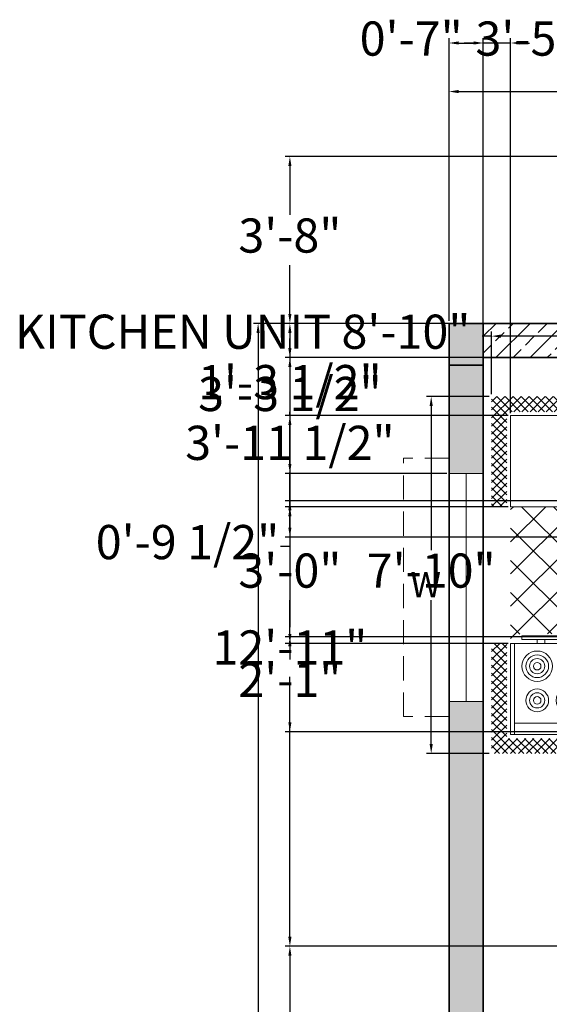
# Model space of a CAD drawing. Units: inches. Extents: x 9689 to 10369, y 10965 to 11626.
# Tile 5 of 11: x 9689 to 9828, y 11359 to 11619. Entities that reach past the tile are written whole.
import ezdxf

# ---------------------------------------------------------------- set-up
doc = ezdxf.new("R2010")
doc.units = ezdxf.units.IN
doc.linetypes.add('DASHED2', pattern=[9.525, 6.35, -3.175])
for name, color, linetype, lineweight in [('A-ANNO-DIMS', 2, 'Continuous', 18), ('A-ANNO-TEXT', 7, 'Continuous', 18), ('A-COLS', 7, 'Continuous', 35), ('A-FLOR-FIXT', 8, 'Continuous', 18), ('A-GLAZ', 4, 'Continuous', 18), ('A-GLAZ-OVHD', 4, 'DASHED2', 13), ('A-WALL', 7, 'Continuous', 35), ('A-WALL-PATT', 252, 'Continuous', 13)]:
    doc.layers.add(name, color=color, linetype=linetype, lineweight=lineweight)
doc.layers.add('A-COLS-PATT', color=18, linetype='Continuous', lineweight=13, true_color=0x000000)
doc.styles.get("Standard").update_dxf_attribs({"font": 'arial.ttf'})
doc.dimstyles.new('ISO-25', dxfattribs={"dimtxt": 9, "dimasz": 2.5, "dimexe": 1.25, "dimexo": 0.625, "dimgap": 2, "dimtad": 0, "dimtih": 1, "dimtoh": 1, "dimdec": 1, "dimlunit": 4, "dimtxsty": 'Standard', "dimcen": 2.5, "dimadec": 0, "dimazin": 0, "dimtfac": 0.5, "dimtdec": 1, "dimtmove": 0, "dimatfit": 3, "dimfxl": 1, "dimarcsym": 0})

# ---------------------------------------------------------------- blocks, each defined once
blk = doc.blocks.new('Kitchen Layout - 7 x 8 ft')
for p, q in [((-5, 81.32), (2.68, 89)), ((-5, 83.44), (0.56, 89)), ((-5, 85.56), (-1.56, 89)), ((-5, 87.68), (-3.68, 89)), ((-1, 84.97), (-5, 88.97)), ((1.09, 85), (-2.91, 89)), ((3.21, 85), (-0.79, 89)), ((0.81, 85), (4.81, 89)), ((5.34, 85), (1.34, 89)), ((2.93, 85), (6.93, 89)), ((7.46, 85), (3.46, 89)), ((5.05, 85), (9.05, 89)), ((9.58, 85), (5.58, 89)), ((7.17, 85), (11.17, 89)), ((11.7, 85), (7.7, 89)), ((9.29, 85), (13.29, 89)), ((13.82, 85), (9.82, 89)), ((11.41, 85), (15.41, 89)), ((15.94, 85), (11.94, 89)), ((13.53, 85), (17.53, 89)), ((18.06, 85), (14.06, 89)), ((15.65, 85), (19.65, 89)), ((20.18, 85), (16.18, 89)), ((17.78, 85), (21.78, 89)), ((22.31, 85), (18.31, 89)), ((19.9, 85), (23.9, 89)), ((24.43, 85), (20.43, 89)), ((22.02, 85), (26.02, 89)), ((26.55, 85), (22.55, 89)), ((24.14, 85), (28.14, 89)), ((28.67, 85), (24.67, 89)), ((26.26, 85), (30.26, 89)), ((30.79, 85), (26.79, 89)), ((28.38, 85), (32.38, 89)), ((32.91, 85), (28.91, 89)), ((30.5, 85), (34.5, 89)), ((35.03, 85), (31.03, 89)), ((32.63, 85), (36.63, 89)), ((37.16, 85), (33.16, 89)), ((34.75, 85), (38.75, 89)), ((39.28, 85), (35.28, 89)), ((36.87, 85), (40.87, 89)), ((41.4, 85), (37.4, 89)), ((38.99, 85), (42.99, 89)), ((43.52, 85), (39.52, 89)), ((41.11, 85), (45.11, 89)), ((45.64, 85), (41.64, 89)), ((43.23, 85), (47.23, 89)), ((47.76, 85), (43.76, 89)), ((45.35, 85), (49.35, 89)), ((49.88, 85), (45.88, 89)), ((47.47, 85), (51.47, 89)), ((52, 85), (48, 89)), ((49.6, 85), (53.6, 89)), ((54.13, 85), (50.13, 89)), ((51.72, 85), (55.72, 89)), ((56.25, 85), (52.25, 89)), ((53.84, 85), (57.84, 89)), ((58.37, 85), (54.37, 89)), ((55.96, 85), (59.96, 89)), ((60.49, 85), (56.49, 89)), ((58.08, 85), (62.08, 89)), ((62.61, 85), (58.61, 89)), ((60.2, 85), (64.2, 89)), ((64.73, 85), (60.73, 89)), ((62.32, 85), (66.32, 89)), ((66.85, 85), (62.85, 89)), ((64.45, 85), (68.45, 89)), ((68.97, 85), (64.97, 89)), ((66.57, 85), (70.57, 89)), ((71.1, 85), (67.1, 89)), ((68.69, 85), (72.69, 89)), ((73.22, 85), (69.22, 89)), ((70.81, 85), (74.81, 89)), ((75.34, 85), (71.34, 89)), ((72.93, 85), (76.93, 89)), ((77.46, 85), (73.46, 89)), ((75.05, 85), (79.05, 89)), ((79.58, 85), (75.58, 89)), ((77.17, 85), (81.17, 89)), ((81.7, 85), (77.7, 89)), ((79.29, 85), (83.29, 89)), ((83.82, 85), (79.82, 89)), ((81.42, 85), (85.42, 89)), ((85.95, 85), (81.95, 89)), ((83.54, 85), (87.54, 89)), ((88.07, 85), (84.07, 89)), ((85.66, 85), (89.66, 89)), ((90.19, 85), (86.19, 89)), ((87.78, 85), (91.78, 89)), ((92.31, 85), (88.31, 89)), ((89.9, 85), (93.9, 89)), ((94.43, 85), (90.43, 89)), ((92.02, 85), (96.02, 89)), ((96.55, 85), (92.55, 89)), ((94.14, 85), (98.14, 89)), ((101, 82.67), (94.67, 89)), ((96.27, 85), (100.27, 89)), ((101, 84.79), (96.79, 89)), ((101, 86.92), (98.92, 89)), ((-1, 82.85), (-5, 86.85)), ((97, 83.61), (101, 87.61)), ((-1, 80.73), (-5, 84.73)), ((-5, 79.19), (-1, 83.19)), ((34, 84), (96, 84)), ((34, 60), (34, 84)), ((96, 84), (96, 60)), ((97, 81.49), (101, 85.49)), ((101, 80.55), (97, 84.55)), ((97, 79.37), (101, 83.37)), ((-1, 78.61), (-5, 82.61)), ((-5, 77.07), (-1, 81.07)), ((-1, 76.49), (-5, 80.49)), ((74, 81), (95, 81)), ((101, 78.43), (97, 82.43)), ((97, 77.25), (101, 81.25)), ((-5, 74.95), (-1, 78.95)), ((-1, 74.36), (-5, 78.36)), ((101, 76.31), (97, 80.31)), ((97, 75.13), (101, 79.13)), ((101, 74.19), (97, 78.19)), ((-5, 72.83), (-1, 76.83)), ((-1, 72.24), (-5, 76.24)), ((97, 73.01), (101, 77.01)), ((101, 72.07), (97, 76.07)), ((-5, 70.71), (-1, 74.71)), ((-1, 70.12), (-5, 74.12)), ((-5, 68.59), (-1, 72.59)), ((97, 70.89), (101, 74.89)), ((101, 69.95), (97, 73.95)), ((97, 68.76), (101, 72.76)), ((-1, 68), (-5, 72)), ((-5, 66.47), (-1, 70.47)), ((101, 67.82), (97, 71.82)), ((97, 66.64), (101, 70.64)), ((-1, 65.88), (-5, 69.88)), ((-5, 64.35), (-1, 68.35)), ((-1, 63.76), (-5, 67.76)), ((101, 65.7), (97, 69.7)), ((97, 64.52), (101, 68.52)), ((101, 63.58), (97, 67.58)), ((-5, 62.22), (-1, 66.22)), ((-1, 61.64), (-5, 65.64)), ((97, 62.4), (101, 66.4)), ((101, 61.46), (97, 65.46)), ((-5, 60.1), (-1, 64.1)), ((-1, 59.52), (-5, 63.52)), ((97, 60.28), (101, 64.28)), ((100.34, 60), (97, 63.34)), ((-5, 57.98), (-1, 61.98)), ((-1, 57.39), (-5, 61.39)), ((-4.86, 56), (-1, 59.86)), ((96, 60), (34, 60)), ((80, 60), (80, 59)), ((82, 59), (82, 60)), ((87, 59), (87, 60)), ((89, 60), (89, 59)), ((98.22, 60), (97, 61.22)), ((98.84, 60), (101, 62.16)), ((100.96, 60), (101, 60.04)), ((-1.73, 56), (-5, 59.27)), ((-3.85, 56), (-5, 57.15)), ((-2.74, 56), (-1, 57.74)), ((10.4, 24), (45.9, 59.5)), ((18.88, 24), (54.38, 59.5)), ((27.37, 24), (62.87, 59.5)), ((33.03, 55.11), (37.41, 59.5)), ((67.71, 24), (33.68, 58.04)), ((35.85, 24), (71.35, 59.5)), ((76.2, 24), (40.7, 59.5)), ((44.34, 24), (77.84, 57.5)), ((84.68, 24), (49.18, 59.5)), ((52.82, 24), (86.32, 57.5)), ((93.17, 24), (57.67, 59.5)), ((61.31, 24), (96, 58.69)), ((96, 29.65), (66.15, 59.5)), ((96, 38.14), (76.64, 57.5)), ((96, 46.63), (85.13, 57.5)), ((96, 55.11), (93.57, 57.54)), ((0, 57), (33, 57)), ((0, 30.57), (24.43, 55)), ((0, 39.06), (15.94, 55)), ((0, 47.54), (7.46, 55)), ((1.91, 24), (32.91, 55)), ((33.77, 24), (2.77, 55)), ((42.26, 24), (11.26, 55)), ((50.74, 24), (19.74, 55)), ((59.23, 24), (28.23, 55)), ((31, 55), (31, 56)), ((32, 55), (31, 55)), ((32, 56), (32, 55)), ((25.29, 24), (0, 49.29)), ((69.79, 24), (96, 50.21)), ((78.28, 24), (96, 41.72)), ((16.8, 24), (0, 40.8)), ((8.32, 24), (0, 32.32)), ((86.76, 24), (96, 33.24)), ((-5, 21.92), (-2.92, 24)), ((-5, 19.8), (-1, 23.8)), ((-1, 21.33), (-3.67, 24)), ((-1, 23.45), (-1.55, 24)), ((0, 24), (96, 24)), ((0, 0), (0, 24)), ((95.25, 24), (96, 24.75)), ((96, 24), (96, 0)), ((97, 22.1), (98.9, 24)), ((97, 19.97), (101, 23.97)), ((101, 21.16), (98.16, 24)), ((101, 23.28), (100.28, 24)), ((-1, 19.21), (-5, 23.21)), ((-5, 17.68), (-1, 21.68)), ((-1, 17.09), (-5, 21.09)), ((101, 19.03), (97, 23.03)), ((97, 17.85), (101, 21.85)), ((101, 16.91), (97, 20.91)), ((-5, 15.55), (-1, 19.55)), ((-1, 14.97), (-5, 18.97)), ((47.25, 6.5), (47.25, 18.5)), ((48.75, 18.5), (48.75, 6.5)), ((97, 15.73), (101, 19.73)), ((101, 14.79), (97, 18.79)), ((-5, 13.43), (-1, 17.43)), ((-1, 12.85), (-5, 16.85)), ((97, 13.61), (101, 17.61)), ((101, 12.67), (97, 16.67)), ((-5, 11.31), (-1, 15.31)), ((-1, 10.73), (-5, 14.73)), ((-5, 9.19), (-1, 13.19)), ((97, 11.49), (101, 15.49)), ((101, 10.55), (97, 14.55)), ((97, 9.37), (101, 13.37)), ((-1, 8.6), (-5, 12.6)), ((-5, 7.07), (-1, 11.07)), ((-1, 6.48), (-5, 10.48)), ((101, 8.43), (97, 12.43)), ((97, 7.25), (101, 11.25)), ((-5, 4.95), (-1, 8.95)), ((-1, 4.36), (-5, 8.36)), ((101, 6.31), (97, 10.31)), ((97, 5.12), (101, 9.12)), ((101, 4.18), (97, 8.18)), ((-5, 2.83), (-1, 6.83)), ((-1, 2.24), (-5, 6.24)), ((97, 3), (101, 7)), ((101, 2.06), (97, 6.06)), ((-5, 0.71), (-1, 4.71)), ((-1, 0.12), (-5, 4.12)), ((64, 4), (32, 4)), ((93.24, -5), (101, 2.76)), ((97, 0.88), (101, 4.88)), ((101, -0.06), (97, 3.94)), ((-5, -1.42), (-1, 2.58)), ((2, -5), (-5, 2)), ((-5, -3.54), (-1, 0.46)), ((96, 0), (0, 0)), ((95.36, -5), (101, 0.64)), ((101, -2.18), (97, 1.82)), ((-0.12, -5), (-5, -0.12)), ((-2.25, -5), (-5, -2.25)), ((-4.34, -5), (-0.34, -1)), ((-2.22, -5), (1.78, -1)), ((-0.1, -5), (3.9, -1)), ((4.12, -5), (0.12, -1)), ((2.02, -5), (6.02, -1)), ((6.24, -5), (2.24, -1)), ((4.14, -5), (8.14, -1)), ((8.36, -5), (4.36, -1)), ((6.27, -5), (10.27, -1)), ((10.48, -5), (6.48, -1)), ((8.39, -5), (12.39, -1)), ((12.6, -5), (8.6, -1)), ((10.51, -5), (14.51, -1)), ((14.73, -5), (10.73, -1)), ((12.63, -5), (16.63, -1)), ((16.85, -5), (12.85, -1)), ((14.75, -5), (18.75, -1)), ((18.97, -5), (14.97, -1)), ((16.87, -5), (20.87, -1)), ((21.09, -5), (17.09, -1)), ((18.99, -5), (22.99, -1)), ((23.21, -5), (19.21, -1)), ((21.11, -5), (25.11, -1)), ((25.33, -5), (21.33, -1)), ((23.24, -5), (27.24, -1)), ((27.45, -5), (23.45, -1)), ((25.36, -5), (29.36, -1)), ((29.57, -5), (25.57, -1)), ((27.48, -5), (30, -2.48)), ((30, -3.3), (27.7, -1)), ((30, -1.18), (29.82, -1)), ((66, -2.54), (67.54, -1)), ((66, -4.66), (69.66, -1)), ((69.88, -5), (66, -1.12)), ((67.78, -5), (71.78, -1)), ((72, -5), (68, -1)), ((69.9, -5), (73.9, -1)), ((74.12, -5), (70.12, -1)), ((72.03, -5), (76.03, -1)), ((76.24, -5), (72.24, -1)), ((74.15, -5), (78.15, -1)), ((78.36, -5), (74.36, -1)), ((76.27, -5), (80.27, -1)), ((80.49, -5), (76.49, -1)), ((78.39, -5), (82.39, -1)), ((82.61, -5), (78.61, -1)), ((80.51, -5), (84.51, -1)), ((84.73, -5), (80.73, -1)), ((82.63, -5), (86.63, -1)), ((86.85, -5), (82.85, -1)), ((84.75, -5), (88.75, -1)), ((88.97, -5), (84.97, -1)), ((86.88, -5), (90.88, -1)), ((91.09, -5), (87.09, -1)), ((89, -5), (93, -1)), ((93.21, -5), (89.21, -1)), ((91.12, -5), (95.12, -1)), ((95.34, -5), (91.34, -1)), ((97.46, -5), (93.46, -1)), ((99.58, -5), (95.58, -1)), ((101, -4.3), (97, -0.3)), ((97.48, -5), (101, -1.48)), ((-4.37, -5), (-5, -4.37)), ((29.6, -5), (30, -4.6)), ((67.76, -5), (66, -3.24)), ((99.6, -5), (101, -3.6))]:
    blk.add_line(p, q)
for points in [[(0, 56), (0, 84), (33, 84), (33, 56)], [(74, 60), (74, 84), (95, 84), (95, 60)], [(76, 58), (76, 59), (93, 59), (93, 58)]]:
    blk.add_lwpolyline(points, close=True)
for points in [[(33.5, 21), (62.5, 21)], [(32, 1.5), (32, 19.5)], [(33.5, 6.5), (33.5, 18.5)], [(34.5, 19.5), (46.25, 19.5)], [(49.75, 19.5), (61.5, 19.5)], [(62.5, 18.5), (62.5, 6.5)], [(64, 19.5), (64, 1.5)], [(46.25, 5.5), (34.5, 5.5)], [(61.5, 5.5), (49.75, 5.5)], [(62.5, 0), (33.5, 0)]]:
    blk.add_lwpolyline(points)
for centre, radius in [((80, 75), 4), ((80, 75), 3), ((89, 75), 3), ((80, 75), 2), ((80, 75), 1), ((89, 75), 2), ((89, 75), 1), ((89, 66), 4), ((80, 66), 3), ((80, 66), 2), ((89, 66), 3), ((89, 66), 2), ((80, 66), 1), ((89, 66), 1), ((40.5, 12.5), 1), ((40.5, 12.5), 0.5), ((55.5, 12.5), 1), ((55.5, 12.5), 0.5)]:
    blk.add_circle(centre, radius)
for centre, radius, start, end in [((33.5, 19.5), 1.5, 90, 180), ((62.5, 19.5), 1.5, 0, 90), ((34.5, 18.5), 1, 90, 180), ((46.25, 18.5), 1, 0, 90), ((49.75, 18.5), 1, 90, 180), ((61.5, 18.5), 1, 0, 90), ((34.5, 6.5), 1, 180, 270), ((46.25, 6.5), 1, 270, 0), ((49.75, 6.5), 1, 180, 270), ((61.5, 6.5), 1, 270, 0), ((33.5, 1.5), 1.5, 180, 270), ((62.5, 1.5), 1.5, 270, 0)]:
    blk.add_arc(centre, radius, start, end)
blk = doc.blocks.new('*D20')
at = {"layer": 'A-ANNO-DIMS', "color": 0, "lineweight": -2, "transparency": 16777216}
for p, q in [((9801.43, 11538.63), (9750.54, 11538.63)), ((9751.79, 11536.13), (9751.79, 11280.15)), ((9751.79, 11011.13), (9751.79, 11267.11)), ((9801.43, 11008.63), (9750.54, 11008.63))]:
    blk.add_line(p, q, dxfattribs=at)
at = {"layer": 'A-ANNO-DIMS', "color": 0, "transparency": 16777216}
for points in [[(9751.38, 11536.13), (9752.21, 11536.13), (9751.79, 11538.63)], [(9751.38, 11011.13), (9752.21, 11011.13), (9751.79, 11008.63)]]:
    blk.add_solid(points, dxfattribs=at)
at = {"layer": 'Defpoints', "color": 0, "transparency": 16777216}
for p in [(9802.06, 11538.63), (9751.79, 11008.63), (9802.06, 11008.63)]:
    blk.add_point(p, dxfattribs=at)
at = {"layer": 'A-ANNO-DIMS', "color": 0, "transparency": 16777216, "insert": (9751.79, 11273.63), "char_height": 9, "attachment_point": 5}
blk.add_mtext('44\'-2"', dxfattribs=at)
blk = doc.blocks.new('*D21')
at = {"layer": 'A-ANNO-DIMS', "color": 0, "lineweight": -2, "transparency": 16777216}
for p, q in [((9802.06, 11539.26), (9802.06, 11600.92)), ((10244.06, 11539.26), (10244.06, 11600.92)), ((9804.56, 11599.67), (10002.11, 11599.67)), ((10241.56, 11599.67), (10044.01, 11599.67))]:
    blk.add_line(p, q, dxfattribs=at)
at = {"layer": 'A-ANNO-DIMS', "color": 0, "transparency": 16777216}
for points in [[(9804.56, 11600.08), (9804.56, 11599.25), (9802.06, 11599.67)], [(10241.56, 11600.08), (10241.56, 11599.25), (10244.06, 11599.67)]]:
    blk.add_solid(points, dxfattribs=at)
at = {"layer": 'Defpoints', "color": 0, "transparency": 16777216}
for p in [(10244.06, 11599.67), (9802.06, 11538.63), (10244.06, 11538.63)]:
    blk.add_point(p, dxfattribs=at)
at = {"layer": 'A-ANNO-DIMS', "color": 0, "transparency": 16777216, "insert": (10023.06, 11599.67), "char_height": 9, "attachment_point": 5}
blk.add_mtext('36\'-10"', dxfattribs=at)
blk = doc.blocks.new('WINDOW-HOOD-68')
for p, q in [((12, 68), (0, 68)), ((0, 0), (0, 68)), ((12, 0), (0, 0))]:
    blk.add_line(p, q)
blk = doc.blocks.new('WINDOW-60')
for p, q in [((0, 60), (9, 60)), ((4.5, 60), (4.5, 0)), ((0, 0), (9, 0))]:
    blk.add_line(p, q)
blk = doc.blocks.new('*D50')
at = {"layer": 'A-ANNO-DIMS', "color": 0, "lineweight": -2, "transparency": 16777216}
for p, q in [((9813.25, 11519.99), (9813.25, 11536.52)), ((9919.25, 11519.99), (9919.25, 11536.52)), ((9813.25, 11535.27), (9810.75, 11535.27)), ((9916.75, 11535.27), (9815.75, 11535.27))]:
    blk.add_line(p, q, dxfattribs=at)
at = {"layer": 'A-ANNO-DIMS', "color": 0, "transparency": 16777216}
for points in [[(9815.75, 11535.69), (9815.75, 11534.85), (9813.25, 11535.27)], [(9916.75, 11535.69), (9916.75, 11534.85), (9919.25, 11535.27)]]:
    blk.add_solid(points, dxfattribs=at)
at = {"layer": 'Defpoints', "color": 0, "transparency": 16777216}
for p in [(9813.25, 11535.27), (9813.25, 11519.37), (9919.25, 11519.37)]:
    blk.add_point(p, dxfattribs=at)
at = {"layer": 'A-ANNO-DIMS', "color": 0, "transparency": 16777216, "insert": (9747.74, 11535.27), "char_height": 9, "attachment_point": 5}
blk.add_mtext('KITCHEN UNIT 8\'-10"', dxfattribs=at)
blk = doc.blocks.new('*D51')
at = {"layer": 'A-ANNO-DIMS', "color": 0, "lineweight": -2, "transparency": 16777216}
for p, q in [((9812.62, 11519.37), (9796.1, 11519.37)), ((9797.35, 11516.87), (9797.35, 11478.96)), ((9797.35, 11427.87), (9797.35, 11465.77)), ((9812.62, 11425.37), (9796.1, 11425.37))]:
    blk.add_line(p, q, dxfattribs=at)
at = {"layer": 'A-ANNO-DIMS', "color": 0, "transparency": 16777216}
for points in [[(9796.93, 11516.87), (9797.77, 11516.87), (9797.35, 11519.37)], [(9796.93, 11427.87), (9797.77, 11427.87), (9797.35, 11425.37)]]:
    blk.add_solid(points, dxfattribs=at)
at = {"layer": 'Defpoints', "color": 0, "transparency": 16777216}
for p in [(9813.25, 11519.37), (9797.35, 11425.37), (9813.25, 11425.37)]:
    blk.add_point(p, dxfattribs=at)
at = {"layer": 'A-ANNO-DIMS', "color": 0, "transparency": 16777216, "insert": (9797.35, 11472.37), "char_height": 9, "attachment_point": 5}
blk.add_mtext('7\'-10"', dxfattribs=at)
blk = doc.blocks.new('*D80')
at = {"layer": 'A-ANNO-DIMS', "color": 0, "lineweight": -2, "transparency": 16777216}
for p, q in [((9979.43, 11529.63), (9758.91, 11529.63)), ((9760.16, 11527.13), (9760.16, 11512.66)), ((9760.16, 11484.88), (9760.16, 11499.35)), ((9979.43, 11482.38), (9758.91, 11482.38))]:
    blk.add_line(p, q, dxfattribs=at)
at = {"layer": 'A-ANNO-DIMS', "color": 0, "transparency": 16777216}
for points in [[(9759.74, 11527.13), (9760.57, 11527.13), (9760.16, 11529.63)], [(9759.74, 11484.88), (9760.57, 11484.88), (9760.16, 11482.38)]]:
    blk.add_solid(points, dxfattribs=at)
at = {"layer": 'Defpoints', "color": 0, "transparency": 16777216}
for p in [(9760.16, 11529.63), (9980.06, 11529.63), (9980.06, 11482.38)]:
    blk.add_point(p, dxfattribs=at)
at = {"layer": 'A-ANNO-DIMS', "color": 0, "transparency": 16777216, "insert": (9760.16, 11506.01), "char_height": 9, "attachment_point": 5}
blk.add_mtext('3\'-11 1/2"', dxfattribs=at)
blk = doc.blocks.new('*D82')
at = {"layer": 'A-ANNO-DIMS', "color": 0, "lineweight": -2, "transparency": 16777216}
for p, q in [((9898.43, 11582.55), (9758.91, 11582.55)), ((9760.16, 11580.05), (9760.16, 11567.19)), ((9760.16, 11541.13), (9760.16, 11553.99)), ((9898.43, 11538.63), (9758.91, 11538.63))]:
    blk.add_line(p, q, dxfattribs=at)
at = {"layer": 'A-ANNO-DIMS', "color": 0, "transparency": 16777216}
for points in [[(9759.74, 11580.05), (9760.57, 11580.05), (9760.16, 11582.55)], [(9759.74, 11541.13), (9760.57, 11541.13), (9760.16, 11538.63)]]:
    blk.add_solid(points, dxfattribs=at)
at = {"layer": 'Defpoints', "color": 0, "transparency": 16777216}
for p in [(9760.16, 11582.55), (9899.06, 11582.55), (9899.06, 11538.63)]:
    blk.add_point(p, dxfattribs=at)
at = {"layer": 'A-ANNO-DIMS', "color": 0, "transparency": 16777216, "insert": (9760.16, 11560.59), "char_height": 9, "attachment_point": 5}
blk.add_mtext('3\'-8"', dxfattribs=at)
blk = doc.blocks.new('*D86')
at = {"layer": 'A-ANNO-DIMS', "color": 0, "lineweight": -2, "transparency": 16777216}
for p, q in [((9802.06, 11539.26), (9802.06, 11613.7)), ((9804.56, 11612.45), (9808.6, 11612.45)), ((9840.56, 11612.45), (9836.52, 11612.45)), ((9843.06, 11539.26), (9843.06, 11613.7))]:
    blk.add_line(p, q, dxfattribs=at)
at = {"layer": 'A-ANNO-DIMS', "color": 0, "transparency": 16777216}
for points in [[(9804.56, 11612.87), (9804.56, 11612.04), (9802.06, 11612.45)], [(9840.56, 11612.87), (9840.56, 11612.04), (9843.06, 11612.45)]]:
    blk.add_solid(points, dxfattribs=at)
at = {"layer": 'Defpoints', "color": 0, "transparency": 16777216}
for p in [(9843.06, 11612.45), (9802.06, 11538.63), (9843.06, 11538.63)]:
    blk.add_point(p, dxfattribs=at)
at = {"layer": 'A-ANNO-DIMS', "color": 0, "transparency": 16777216, "insert": (9822.56, 11612.45), "char_height": 9, "attachment_point": 5}
blk.add_mtext('3\'-5"', dxfattribs=at)
blk = doc.blocks.new('*D91')
at = {"layer": 'A-ANNO-DIMS', "color": 0, "lineweight": -2, "transparency": 16777216}
for p, q in [((9801.43, 11538.63), (9758.91, 11538.63)), ((9760.16, 11536.13), (9760.16, 11525.53)), ((9760.16, 11501.61), (9760.16, 11512.22)), ((9801.43, 11499.11), (9758.91, 11499.11))]:
    blk.add_line(p, q, dxfattribs=at)
at = {"layer": 'A-ANNO-DIMS', "color": 0, "transparency": 16777216}
for points in [[(9759.74, 11536.13), (9760.57, 11536.13), (9760.16, 11538.63)], [(9759.74, 11501.61), (9760.57, 11501.61), (9760.16, 11499.11)]]:
    blk.add_solid(points, dxfattribs=at)
at = {"layer": 'Defpoints', "color": 0, "transparency": 16777216}
for p in [(9760.16, 11538.63), (9802.06, 11538.63), (9802.06, 11499.11)]:
    blk.add_point(p, dxfattribs=at)
at = {"layer": 'A-ANNO-DIMS', "color": 0, "transparency": 16777216, "insert": (9760.16, 11518.87), "char_height": 9, "attachment_point": 5}
blk.add_mtext('3\'-3 1/2"', dxfattribs=at)
blk = doc.blocks.new('*D99')
at = {"layer": 'A-ANNO-DIMS', "color": 0, "lineweight": -2, "transparency": 16777216}
for p, q in [((9922.43, 11374.63), (9758.91, 11374.63)), ((9760.16, 11372.13), (9760.16, 11357.23)), ((9760.16, 11329.13), (9760.16, 11344.03)), ((9801.43, 11326.63), (9758.91, 11326.63))]:
    blk.add_line(p, q, dxfattribs=at)
at = {"layer": 'A-ANNO-DIMS', "color": 0, "transparency": 16777216}
for points in [[(9759.74, 11372.13), (9760.57, 11372.13), (9760.16, 11374.63)], [(9759.74, 11329.13), (9760.57, 11329.13), (9760.16, 11326.63)]]:
    blk.add_solid(points, dxfattribs=at)
at = {"layer": 'Defpoints', "color": 0, "transparency": 16777216}
for p in [(9923.06, 11374.63), (9760.16, 11326.63), (9802.06, 11326.63)]:
    blk.add_point(p, dxfattribs=at)
at = {"layer": 'A-ANNO-DIMS', "color": 0, "transparency": 16777216, "insert": (9760.16, 11350.63), "char_height": 9, "attachment_point": 5}
blk.add_mtext('4\'-0"', dxfattribs=at)
blk = doc.blocks.new('*D108')
at = {"layer": 'A-ANNO-DIMS', "color": 0, "lineweight": -2, "transparency": 16777216}
for p, q in [((9922.43, 11529.63), (9758.91, 11529.63)), ((9760.16, 11527.13), (9760.16, 11458.65)), ((9760.16, 11377.13), (9760.16, 11445.61)), ((9922.43, 11374.63), (9758.91, 11374.63))]:
    blk.add_line(p, q, dxfattribs=at)
at = {"layer": 'A-ANNO-DIMS', "color": 0, "transparency": 16777216}
for points in [[(9759.74, 11527.13), (9760.57, 11527.13), (9760.16, 11529.63)], [(9759.74, 11377.13), (9760.57, 11377.13), (9760.16, 11374.63)]]:
    blk.add_solid(points, dxfattribs=at)
at = {"layer": 'Defpoints', "color": 0, "transparency": 16777216}
for p in [(9760.16, 11529.63), (9923.06, 11529.63), (9923.06, 11374.63)]:
    blk.add_point(p, dxfattribs=at)
at = {"layer": 'A-ANNO-DIMS', "color": 0, "transparency": 16777216, "insert": (9760.16, 11452.13), "char_height": 9, "attachment_point": 5}
blk.add_mtext('12\'-11"', dxfattribs=at)
blk = doc.blocks.new('*D110')
at = {"layer": 'A-ANNO-DIMS', "color": 0, "lineweight": -2, "transparency": 16777216}
for p, q in [((10021.43, 11456.13), (9758.91, 11456.13)), ((9760.16, 11453.63), (9760.16, 11450.15)), ((9760.16, 11433.63), (9760.16, 11437.11)), ((10021.43, 11431.13), (9758.91, 11431.13))]:
    blk.add_line(p, q, dxfattribs=at)
at = {"layer": 'A-ANNO-DIMS', "color": 0, "transparency": 16777216}
for points in [[(9759.74, 11453.63), (9760.57, 11453.63), (9760.16, 11456.13)], [(9759.74, 11433.63), (9760.57, 11433.63), (9760.16, 11431.13)]]:
    blk.add_solid(points, dxfattribs=at)
at = {"layer": 'Defpoints', "color": 0, "transparency": 16777216}
for p in [(9760.16, 11456.13), (10022.06, 11456.13), (10022.06, 11431.13)]:
    blk.add_point(p, dxfattribs=at)
at = {"layer": 'A-ANNO-DIMS', "color": 0, "transparency": 16777216, "insert": (9760.16, 11443.63), "char_height": 9, "attachment_point": 5}
blk.add_mtext('2\'-1"', dxfattribs=at)
blk = doc.blocks.new('*D114')
at = {"layer": 'A-ANNO-DIMS', "color": 0, "lineweight": -2, "transparency": 16777216}
for p, q in [((9817.62, 11490.37), (9758.91, 11490.37)), ((9760.16, 11487.87), (9760.16, 11478.97)), ((9760.16, 11456.87), (9760.16, 11465.77)), ((9817.62, 11454.37), (9758.91, 11454.37))]:
    blk.add_line(p, q, dxfattribs=at)
at = {"layer": 'A-ANNO-DIMS', "color": 0, "transparency": 16777216}
for points in [[(9759.74, 11487.87), (9760.57, 11487.87), (9760.16, 11490.37)], [(9759.74, 11456.87), (9760.57, 11456.87), (9760.16, 11454.37)]]:
    blk.add_solid(points, dxfattribs=at)
at = {"layer": 'Defpoints', "color": 0, "transparency": 16777216}
for p in [(9760.16, 11490.37), (9818.25, 11490.37), (9818.25, 11454.37)]:
    blk.add_point(p, dxfattribs=at)
at = {"layer": 'A-ANNO-DIMS', "color": 0, "transparency": 16777216, "insert": (9760.16, 11472.37), "char_height": 9, "attachment_point": 5}
blk.add_mtext('3\'-0"', dxfattribs=at)
blk = doc.blocks.new('*D115')
at = {"layer": 'A-ANNO-DIMS', "color": 0, "lineweight": -2, "transparency": 16777216}
for p, q in [((9760.16, 11532.13), (9760.16, 11534.63)), ((9810.43, 11529.63), (9758.91, 11529.63)), ((9760.16, 11529.63), (9760.16, 11528.66)), ((9817.62, 11514.37), (9758.91, 11514.37)), ((9760.16, 11514.37), (9760.16, 11515.34)), ((9760.16, 11511.87), (9760.16, 11509.37))]:
    blk.add_line(p, q, dxfattribs=at)
at = {"layer": 'A-ANNO-DIMS', "color": 0, "transparency": 16777216}
for points in [[(9759.74, 11532.13), (9760.57, 11532.13), (9760.16, 11529.63)], [(9759.74, 11511.87), (9760.57, 11511.87), (9760.16, 11514.37)]]:
    blk.add_solid(points, dxfattribs=at)
at = {"layer": 'Defpoints', "color": 0, "transparency": 16777216}
for p in [(9760.16, 11529.63), (9811.06, 11529.63), (9818.25, 11514.37)]:
    blk.add_point(p, dxfattribs=at)
at = {"layer": 'A-ANNO-DIMS', "color": 0, "transparency": 16777216, "insert": (9760.16, 11522), "char_height": 9, "attachment_point": 5}
blk.add_mtext('1\'-3 1/2"', dxfattribs=at)
blk = doc.blocks.new('*D116')
at = {"layer": 'A-ANNO-DIMS', "color": 0, "lineweight": -2, "transparency": 16777216}
for p, q in [((9808.56, 11612.45), (9806.06, 11612.45)), ((9811.06, 11530.26), (9811.06, 11613.7)), ((9818.25, 11612.45), (9811.06, 11612.45)), ((9818.25, 11514.99), (9818.25, 11613.7)), ((9820.75, 11612.45), (9823.25, 11612.45))]:
    blk.add_line(p, q, dxfattribs=at)
at = {"layer": 'A-ANNO-DIMS', "color": 0, "transparency": 16777216}
for points in [[(9808.56, 11612.87), (9808.56, 11612.04), (9811.06, 11612.45)], [(9820.75, 11612.87), (9820.75, 11612.04), (9818.25, 11612.45)]]:
    blk.add_solid(points, dxfattribs=at)
at = {"layer": 'Defpoints', "color": 0, "transparency": 16777216}
for p in [(9811.06, 11612.45), (9811.06, 11529.63), (9818.25, 11514.37)]:
    blk.add_point(p, dxfattribs=at)
at = {"layer": 'A-ANNO-DIMS', "color": 0, "transparency": 16777216, "insert": (9792.09, 11612.45), "char_height": 9, "attachment_point": 5}
blk.add_mtext('0\'-7"', dxfattribs=at)
blk = doc.blocks.new('*D118')
at = {"layer": 'A-ANNO-DIMS', "color": 0, "lineweight": -2, "transparency": 16777216}
for p, q in [((9980.91, 11491.91), (9758.91, 11491.91)), ((9760.16, 11489.41), (9760.16, 11484.88)), ((9979.43, 11482.38), (9758.91, 11482.38)), ((9760.16, 11482.38), (9760.16, 11479.88)), ((9760.16, 11479.88), (9757.66, 11479.88))]:
    blk.add_line(p, q, dxfattribs=at)
at = {"layer": 'A-ANNO-DIMS', "color": 0, "transparency": 16777216}
for points in [[(9759.74, 11489.41), (9760.57, 11489.41), (9760.16, 11491.91)], [(9759.74, 11484.88), (9760.57, 11484.88), (9760.16, 11482.38)]]:
    blk.add_solid(points, dxfattribs=at)
at = {"layer": 'Defpoints', "color": 0, "transparency": 16777216}
for p in [(9981.53, 11491.91), (9760.16, 11482.38), (9980.06, 11482.38)]:
    blk.add_point(p, dxfattribs=at)
at = {"layer": 'A-ANNO-DIMS', "color": 0, "transparency": 16777216, "insert": (9733.21, 11479.88), "char_height": 9, "attachment_point": 5}
blk.add_mtext('0\'-9 1/2"', dxfattribs=at)

msp = doc.modelspace()

# ---------------------------------------------------------------- hatches: boundary and pattern name
at = {"layer": 'A-COLS-PATT'}
h = msp.add_hatch(color=256, dxfattribs=at)
h.dxf.hatch_style = 1
h.paths.add_polyline_path([(9811.06, 11538.63), (9802.06, 11538.63), (9802.06, 11527.63), (9811.06, 11527.63), (9811.06, 11529.63)])
at = {"layer": 'A-WALL-PATT'}
h = msp.add_hatch(dxfattribs=at)
h.set_pattern_fill('ANSI33', color=256)
h.paths.add_polyline_path([(9843.06, 11538.63), (9811.06, 11538.63), (9811.06, 11529.63), (9843.06, 11529.63)])
h.paths.add_polyline_path([(9923.06, 11538.63), (9891.06, 11538.63), (9891.06, 11529.63), (9923.06, 11529.63)])
h.paths.add_polyline_path([(9929.06, 11527.63), (9923.06, 11527.63), (9923.06, 11380.63), (9929.06, 11380.63)])
h.paths.add_polyline_path([(9939.06, 11538.63), (9929.06, 11538.63), (9929.06, 11529.63), (9939.06, 11529.63, -0.071068)])
h.paths.add_polyline_path([(10035.06, 11538.63), (10013.06, 11538.63), (10013.06, 11529.63), (10022.06, 11529.63), (10022.06, 11507.38), (10022.06, 11502.38), (10022.06, 11482.38), (10022.06, 11478.38), (10022.06, 11456.13, -0.038405), (10026.06, 11456.13), (10026.06, 11502.38), (10026.06, 11529.63), (10035.06, 11529.63)])
h.paths.add_polyline_path([(10068.06, 11538.63), (10059.06, 11538.63), (10059.06, 11529.63), (10068.06, 11529.63)])
h.paths.add_polyline_path([(10074.06, 11527.63), (10068.06, 11527.63), (10068.06, 11431.13), (10026.06, 11431.13), (10022.06, 11431.13), (9980.06, 11431.13), (9976.06, 11431.13), (9976.06, 11425.13), (10068.06, 11425.13), (10068.06, 11380.63), (10074.06, 11380.63)])
h.paths.add_polyline_path([(10124.56, 11538.63), (10074.06, 11538.63), (10074.06, 11529.63), (10124.56, 11529.63)])
h.paths.add_polyline_path([(9980.06, 11507.38), (9980.06, 11529.63), (9989.06, 11529.63), (9989.06, 11538.63), (9976.06, 11538.63), (9976.06, 11529.63), (9976.06, 11503.38), (9976.06, 11483.38), (9976.06, 11478.38), (9980.06, 11478.38), (9997.06, 11478.38, -0.038405), (9997.06, 11482.38), (9980.06, 11482.38)])
h.paths.add_polyline_path([(10235.06, 11538.63), (10184.56, 11538.63), (10184.56, 11529.63), (10235.06, 11529.63)])
h.paths.add_polyline_path([(10244.06, 11527.63), (10235.06, 11527.63), (10235.06, 11485.13), (10244.06, 11485.13)])
h.paths.add_polyline_path([(10244.06, 11425.13), (10235.06, 11425.13), (10235.06, 11380.63), (10244.06, 11380.63)])
h.paths.add_polyline_path([(10233.06, 11380.63), (10120.06, 11380.63, -0.038405), (10120.06, 11374.63), (10133.04, 11374.63), (10133.04, 11326.63), (10120.06, 11326.63, -0.038405), (10120.06, 11320.63), (10149.19, 11320.63), (10149.19, 11326.63), (10136.04, 11326.63), (10136.04, 11374.63), (10233.06, 11374.63)])
h.paths.add_polyline_path([(10084.06, 11380.63), (10076.06, 11380.63), (10076.06, 11374.63), (10084.06, 11374.63)])
h.paths.add_polyline_path([(10244.06, 11374.63), (10235.06, 11374.63), (10235.06, 11362.63), (10244.06, 11362.63)])
h.paths.add_polyline_path([(10244.06, 11338.63), (10235.06, 11338.63), (10235.06, 11326.63), (10244.06, 11326.63)])
h.paths.add_polyline_path([(10233.06, 11326.63), (10173.19, 11326.63, -0.055385), (10173.19, 11320.63), (10233.06, 11320.63)], flags=0)
h.paths.add_polyline_path([(10244.06, 11320.63), (10235.06, 11320.63), (10235.06, 11273.63), (10244.06, 11273.63)])
h = msp.add_hatch(dxfattribs=at)
h.set_pattern_fill('ANSI36', color=256)
h.paths.add_polyline_path([(10233.06, 11326.63), (10173.19, 11326.63, -0.055385), (10173.19, 11320.63), (10233.06, 11320.63)])
h.paths.add_polyline_path([(10244.06, 11213.63), (10235.06, 11213.63), (10235.06, 11166.63), (10244.06, 11166.63)])
h.paths.add_polyline_path([(10233.06, 11166.63), (10184.56, 11166.63), (10184.56, 11157.63), (10233.06, 11157.63)])
h.paths.add_polyline_path([(10124.56, 11166.63), (10074.06, 11166.63), (10074.06, 11157.63), (10124.56, 11157.63)])
h.paths.add_polyline_path([(10074.06, 11318.63), (10068.06, 11318.63), (10068.06, 11168.63), (10074.06, 11168.63)])
h.paths.add_polyline_path([(10068.06, 11166.63), (10011.06, 11166.63), (10011.06, 11157.63), (10068.06, 11157.63)])
h.paths.add_polyline_path([(10011.06, 11318.63), (10005.06, 11318.63), (10005.06, 11168.63), (10011.06, 11168.63)])
h.paths.add_polyline_path([(10005.06, 11166.63), (9985.06, 11166.63), (9985.06, 11157.63), (10005.06, 11157.63)])
h.paths.add_polyline_path([(9937.06, 11166.63), (9898.06, 11166.63), (9898.06, 11157.63), (9937.06, 11157.63, -0.042779)])
h.paths.add_polyline_path([(9850.06, 11166.63), (9813.06, 11166.63), (9813.06, 11157.63), (9850.06, 11157.63)])
h.paths.add_polyline_path([(9811.06, 11213.63), (9802.06, 11213.63), (9802.06, 11166.63), (9811.06, 11166.63)])
h.paths.add_polyline_path([(9811.06, 11320.63), (9802.06, 11320.63), (9802.06, 11273.63), (9811.06, 11273.63)])
h.paths.add_polyline_path([(9811.06, 11439.11), (9802.06, 11439.11), (9802.06, 11326.63), (9811.06, 11326.63)])
h.paths.add_polyline_path([(9957.06, 11326.63), (9813.06, 11326.63), (9813.06, 11320.63), (9957.06, 11320.63)])
h.paths.add_polyline_path([(9811.06, 11527.63), (9802.06, 11527.63), (9802.06, 11499.11), (9811.06, 11499.11)])

# ---------------------------------------------------------------- linework, layer by layer
at = {"layer": 'A-COLS'}
for p, q in [((9811.06, 11529.63), (9811.06, 11538.63)), ((9811.06, 11527.63), (9802.06, 11527.63))]:
    msp.add_line(p, q, dxfattribs=at)
at = {"layer": 'A-GLAZ'}
msp.add_line((9811.06, 11499.11), (9811.06, 11439.11), dxfattribs=at)
at = {"layer": 'A-WALL'}
for p, q in [((9802.06, 11538.63), (9939.06, 11538.63)), ((9802.06, 11157.63), (9802.06, 11538.63)), ((9811.06, 11529.63), (9923.06, 11529.63)), ((9811.06, 11326.63), (9811.06, 11529.63))]:
    msp.add_line(p, q, dxfattribs=at)

# ---------------------------------------------------------------- block references
at = {"layer": 'A-FLOR-FIXT', "rotation": 180}
msp.add_blockref('Kitchen Layout - 7 x 8 ft', (9914.25, 11514.37), dxfattribs=at)
at = {"layer": 'A-GLAZ'}
msp.add_blockref('WINDOW-60', (9802.06, 11439.11), dxfattribs=at)
at = {"layer": 'A-GLAZ-OVHD'}
msp.add_blockref('WINDOW-HOOD-68', (9790.06, 11435.11), dxfattribs=at)

# ---------------------------------------------------------------- texts
at = {"layer": 'A-ANNO-TEXT', "insert": (9791.89, 11473.21), "char_height": 6.729, "attachment_point": 1}
msp.add_mtext_dynamic_manual_height_columns('{\\fArial|b1|i0|c0|p34;W}', width=31.3623, gutter_width=33.65, heights=[0], dxfattribs=at)

# ---------------------------------------------------------------- dimensions: what is measured, and where the dimension line sits
at = {"layer": 'A-ANNO-DIMS'}
for base, p1, p2, override, picture, middle in [((9811.06, 11612.45), (9818.25, 11514.37), (9811.06, 11529.63), {"dimdec": 1, "dimlfac": 1, "dimrnd": 0, "dimzin": 1, "dimdsep": 46, "dimlunit": 4, "dimfrac": 2}, '*D116', (9792.09, 11612.45)), ((9843.06, 11612.45), (9802.06, 11538.63), (9843.06, 11538.63), {"dimdec": 1, "dimlfac": 1, "dimrnd": 0, "dimzin": 1, "dimdsep": 46, "dimlunit": 4, "dimfrac": 2}, '*D86', (9822.56, 11612.45)), ((10244.06, 11599.67), (9802.06, 11538.63), (10244.06, 11538.63), {"dimclrd": 0, "dimclre": 0, "dimclrt": 0}, '*D21', (10023.06, 11599.67))]:
    dim = msp.add_linear_dim(base=base, p1=p1, p2=p2, dimstyle='ISO-25', override=override, dxfattribs=at)
    dim.commit()
    dim.dimension.update_dxf_attribs({"geometry": picture, "text_midpoint": middle})
for base, p1, p2, angle, override, picture, middle in [((9760.16, 11582.55), (9899.06, 11538.63), (9899.06, 11582.55), 90, {"dimdec": 1, "dimlfac": 1, "dimrnd": 0, "dimzin": 1, "dimdsep": 46, "dimlunit": 4, "dimfrac": 2}, '*D82', (9760.16, 11560.59)), ((9751.79, 11008.63), (9802.06, 11538.63), (9802.06, 11008.63), 90, {"dimclrd": 0, "dimclre": 0, "dimclrt": 0}, '*D20', (9751.79, 11273.63)), ((9760.16, 11538.63), (9802.06, 11499.11), (9802.06, 11538.63), 90, {"dimdec": 1, "dimlfac": 1, "dimrnd": 0, "dimzin": 1, "dimdsep": 46, "dimlunit": 4, "dimfrac": 2}, '*D91', (9760.16, 11518.87)), ((9760.16, 11529.63), (9818.25, 11514.37), (9811.06, 11529.63), 90, {"dimdec": 1, "dimlfac": 1, "dimrnd": 0, "dimzin": 1, "dimdsep": 46, "dimlunit": 4, "dimfrac": 2}, '*D115', (9760.16, 11522)), ((9760.15676, 11529.630116), (9980.05676, 11482.380116), (9980.05676, 11529.630116), 90, {"dimdec": 1, "dimlfac": 1, "dimrnd": 0, "dimzin": 1, "dimdsep": 46, "dimlunit": 4, "dimfrac": 2}, '*D80', (9760.15676, 11506.005116)), ((9760.16, 11529.63), (9923.06, 11374.63), (9923.06, 11529.63), 90, {"dimdec": 1, "dimlfac": 1, "dimrnd": 0, "dimzin": 1, "dimdsep": 46, "dimlunit": 4, "dimfrac": 2}, '*D108', (9760.16, 11452.13)), ((9797.35, 11425.37), (9813.25, 11519.37), (9813.25, 11425.37), 270, {"dimdec": 1, "dimlfac": 1, "dimrnd": 0, "dimzin": 1, "dimdsep": 46, "dimlunit": 4, "dimfrac": 2}, '*D51', (9797.35, 11472.37)), ((9760.16, 11482.38), (9981.53, 11491.91), (9980.06, 11482.38), 90, {"dimdec": 1, "dimlfac": 1, "dimrnd": 0, "dimzin": 1, "dimdsep": 46, "dimlunit": 4, "dimfrac": 2}, '*D118', (9733.21, 11479.88)), ((9760.16, 11490.37), (9818.25, 11454.37), (9818.25, 11490.37), 90, {"dimdec": 1, "dimlfac": 1, "dimrnd": 0, "dimzin": 1, "dimdsep": 46, "dimlunit": 4, "dimfrac": 2}, '*D114', (9760.16, 11472.37)), ((9760.16, 11456.13), (10022.06, 11431.13), (10022.06, 11456.13), 90, {"dimdec": 1, "dimlfac": 1, "dimrnd": 0, "dimzin": 1, "dimdsep": 46, "dimlunit": 4, "dimfrac": 2}, '*D110', (9760.16, 11443.63)), ((9760.16, 11326.63), (9923.06, 11374.63), (9802.06, 11326.63), 90, {"dimdec": 1, "dimlfac": 1, "dimrnd": 0, "dimzin": 1, "dimdsep": 46, "dimlunit": 4, "dimfrac": 2}, '*D99', (9760.16, 11350.63))]:
    dim = msp.add_linear_dim(base=base, p1=p1, p2=p2, angle=angle, dimstyle='ISO-25', override=override, dxfattribs=at)
    dim.commit()
    dim.dimension.update_dxf_attribs({"geometry": picture, "text_midpoint": middle})
dim = msp.add_linear_dim(base=(9813.25, 11535.27), p1=(9919.25, 11519.37), p2=(9813.25, 11519.37), angle=180, text='KITCHEN UNIT <>', dimstyle='ISO-25', override={"dimdec": 1, "dimlfac": 1, "dimrnd": 0, "dimzin": 1, "dimdsep": 46, "dimlunit": 4, "dimfrac": 2}, dxfattribs=at)
dim.commit()
dim.dimension.update_dxf_attribs({"geometry": '*D50', "text_midpoint": (9747.74, 11535.27)})

doc.saveas('drawing.dxf')
